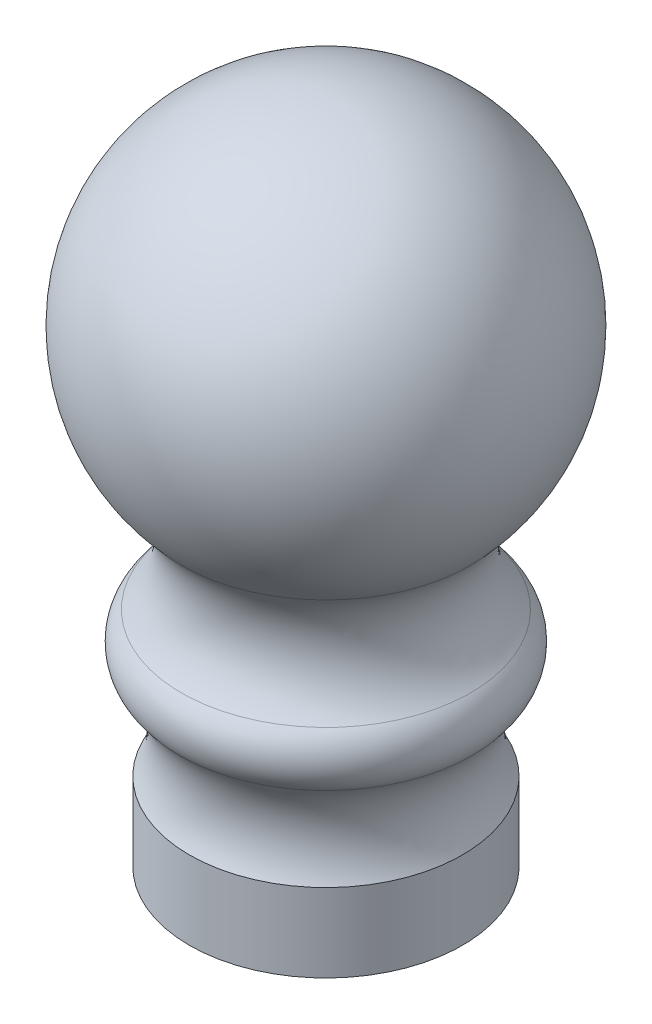
ISO-10303-21;
HEADER;
FILE_DESCRIPTION(('STEP AP214'),'2;1');
FILE_NAME('part.step','',(''),(''),'','','');
FILE_SCHEMA(('AUTOMOTIVE_DESIGN { 1 0 10303 214 1 1 1 1 }'));
ENDSEC;
DATA;
#1=APPLICATION_CONTEXT('core data for automotive mechanical design processes');
#2=APPLICATION_PROTOCOL_DEFINITION('international standard','automotive_design',2000,#1);
#3=PRODUCT_CONTEXT('',#1,'mechanical');
#4=PRODUCT('Part','Part','',(#3));
#5=PRODUCT_RELATED_PRODUCT_CATEGORY('part','',(#4));
#6=PRODUCT_DEFINITION_FORMATION('','',#4);
#7=PRODUCT_DEFINITION_CONTEXT('part definition',#1,'design');
#8=PRODUCT_DEFINITION('design','',#6,#7);
#9=PRODUCT_DEFINITION_SHAPE('','',#8);
#10=(LENGTH_UNIT() NAMED_UNIT(*) SI_UNIT(.MILLI.,.METRE.));
#11=(NAMED_UNIT(*) PLANE_ANGLE_UNIT() SI_UNIT($,.RADIAN.));
#12=(NAMED_UNIT(*) SI_UNIT($,.STERADIAN.) SOLID_ANGLE_UNIT());
#13=UNCERTAINTY_MEASURE_WITH_UNIT(LENGTH_MEASURE(1.E-05),#10,'distance_accuracy_value','');
#14=(GEOMETRIC_REPRESENTATION_CONTEXT(3) GLOBAL_UNCERTAINTY_ASSIGNED_CONTEXT((#13)) GLOBAL_UNIT_ASSIGNED_CONTEXT((#10,
#11,#12)) REPRESENTATION_CONTEXT('',''));
#15=CARTESIAN_POINT('',(0.,0.,0.));
#16=DIRECTION('',(0.,0.,1.));
#17=DIRECTION('',(1.,0.,0.));
#18=AXIS2_PLACEMENT_3D('',#15,#16,#17);
#19=CARTESIAN_POINT('',(0.,24.,0.));
#20=DIRECTION('',(0.,-1.,0.));
#21=DIRECTION('',(1.,0.,0.));
#22=AXIS2_PLACEMENT_3D('',#19,#20,#21);
#23=SPHERICAL_SURFACE('',#22,10.147938904834);
#24=CARTESIAN_POINT('',(0.,24.,-9.32634247796231));
#25=DIRECTION('',(0.,0.,1.));
#26=DIRECTION('',(1.,0.,0.));
#27=AXIS2_PLACEMENT_3D('',#24,#25,#26);
#28=CIRCLE('',#27,4.);
#29=CARTESIAN_POINT('',(4.,24.,-9.32634247796231));
#30=VERTEX_POINT('',#29);
#31=EDGE_CURVE('E44',#30,#30,#28,.T.);
#32=ORIENTED_EDGE('',*,*,#31,.T.);
#33=EDGE_LOOP('',(#32));
#34=FACE_BOUND('',#33,.T.);
#35=CARTESIAN_POINT('',(0.,17.0710678118655,0.));
#36=DIRECTION('',(0.,-1.,0.));
#37=DIRECTION('',(0.,0.,-1.));
#38=AXIS2_PLACEMENT_3D('',#35,#36,#37);
#39=CIRCLE('',#38,7.4142135623731);
#40=CARTESIAN_POINT('',(0.,17.0710678118655,-7.4142135623731));
#41=VERTEX_POINT('',#40);
#42=EDGE_CURVE('E11',#41,#41,#39,.T.);
#43=ORIENTED_EDGE('',*,*,#42,.F.);
#44=EDGE_LOOP('',(#43));
#45=FACE_BOUND('',#44,.T.);
#46=CARTESIAN_POINT('',(-9.32634247796231,24.,0.));
#47=DIRECTION('',(1.,0.,0.));
#48=DIRECTION('',(0.,0.,-1.));
#49=AXIS2_PLACEMENT_3D('',#46,#47,#48);
#50=CIRCLE('',#49,4.);
#51=CARTESIAN_POINT('',(-9.32634247796231,24.,-4.));
#52=VERTEX_POINT('',#51);
#53=EDGE_CURVE('E98',#52,#52,#50,.T.);
#54=ORIENTED_EDGE('',*,*,#53,.T.);
#55=EDGE_LOOP('',(#54));
#56=FACE_BOUND('',#55,.T.);
#57=ADVANCED_FACE('F41',(#34,#45,#56),#23,.T.);
#58=CARTESIAN_POINT('',(0.,24.,4.));
#59=DIRECTION('',(0.,0.,-1.));
#60=DIRECTION('',(-1.,0.,0.));
#61=AXIS2_PLACEMENT_3D('',#58,#59,#60);
#62=CYLINDRICAL_SURFACE('',#61,4.);
#63=ORIENTED_EDGE('',*,*,#31,.F.);
#64=EDGE_LOOP('',(#63));
#65=FACE_BOUND('',#64,.T.);
#66=CARTESIAN_POINT('',(0.,24.,0.));
#67=DIRECTION('',(0.707106781186547,0.,-0.707106781186547));
#68=DIRECTION('',(-0.707106781186547,0.,-0.707106781186547));
#69=AXIS2_PLACEMENT_3D('',#66,#67,#68);
#70=ELLIPSE('',#69,5.65685424949238,4.);
#71=CARTESIAN_POINT('',(0.,28.,0.));
#72=VERTEX_POINT('',#71);
#73=CARTESIAN_POINT('',(0.,20.,0.));
#74=VERTEX_POINT('',#73);
#75=EDGE_CURVE('E60',#72,#74,#70,.F.);
#76=ORIENTED_EDGE('',*,*,#75,.T.);
#77=CARTESIAN_POINT('',(0.,24.,0.));
#78=DIRECTION('',(-0.707106781186547,0.,-0.707106781186547));
#79=DIRECTION('',(0.707106781186547,0.,-0.707106781186547));
#80=AXIS2_PLACEMENT_3D('',#77,#78,#79);
#81=ELLIPSE('',#80,5.65685424949238,4.);
#82=CARTESIAN_POINT('',(4.,24.,-4.));
#83=VERTEX_POINT('',#82);
#84=EDGE_CURVE('E76',#74,#83,#81,.F.);
#85=ORIENTED_EDGE('',*,*,#84,.T.);
#86=EDGE_CURVE('E71',#83,#72,#81,.F.);
#87=ORIENTED_EDGE('',*,*,#86,.T.);
#88=EDGE_LOOP('',(#76,#85,#87));
#89=FACE_BOUND('',#88,.T.);
#90=ADVANCED_FACE('F95',(#65,#89),#62,.F.);
#91=CARTESIAN_POINT('',(0.,14.2426406871193,0.));
#92=DIRECTION('',(0.,-1.,0.));
#93=DIRECTION('',(0.,0.,-1.));
#94=AXIS2_PLACEMENT_3D('',#91,#92,#93);
#95=TOROIDAL_SURFACE('',#94,10.2426406871193,4.);
#96=ORIENTED_EDGE('',*,*,#42,.T.);
#97=EDGE_LOOP('',(#96));
#98=FACE_BOUND('',#97,.T.);
#99=CARTESIAN_POINT('',(0.,11.4142135623731,0.));
#100=DIRECTION('',(0.,-1.,0.));
#101=DIRECTION('',(0.,0.,-1.));
#102=AXIS2_PLACEMENT_3D('',#99,#100,#101);
#103=CIRCLE('',#102,7.4142135623731);
#104=CARTESIAN_POINT('',(0.,11.4142135623731,-7.4142135623731));
#105=VERTEX_POINT('',#104);
#106=EDGE_CURVE('E104',#105,#105,#103,.T.);
#107=ORIENTED_EDGE('',*,*,#106,.F.);
#108=EDGE_LOOP('',(#107));
#109=FACE_BOUND('',#108,.T.);
#110=ADVANCED_FACE('F43',(#98,#109),#95,.F.);
#111=CARTESIAN_POINT('',(0.,0.,0.));
#112=DIRECTION('',(0.,-1.,0.));
#113=DIRECTION('',(0.,0.,-1.));
#114=AXIS2_PLACEMENT_3D('',#111,#112,#113);
#115=PLANE('',#114);
#116=CARTESIAN_POINT('',(0.,0.,0.));
#117=DIRECTION('',(0.,-1.,0.));
#118=DIRECTION('',(0.,0.,-1.));
#119=AXIS2_PLACEMENT_3D('',#116,#117,#118);
#120=CIRCLE('',#119,7.);
#121=CARTESIAN_POINT('',(0.,0.,-7.));
#122=VERTEX_POINT('',#121);
#123=EDGE_CURVE('E49',#122,#122,#120,.T.);
#124=ORIENTED_EDGE('',*,*,#123,.T.);
#125=EDGE_LOOP('',(#124));
#126=FACE_BOUND('',#125,.T.);
#127=ADVANCED_FACE('F119',(#126),#115,.T.);
#128=CARTESIAN_POINT('',(0.,0.,0.));
#129=DIRECTION('',(0.,-1.,0.));
#130=DIRECTION('',(0.,0.,-1.));
#131=AXIS2_PLACEMENT_3D('',#128,#129,#130);
#132=CYLINDRICAL_SURFACE('',#131,7.);
#133=CARTESIAN_POINT('',(0.,4.01398088881321,0.));
#134=DIRECTION('',(0.,-1.,0.));
#135=DIRECTION('',(0.,0.,-1.));
#136=AXIS2_PLACEMENT_3D('',#133,#134,#135);
#137=CIRCLE('',#136,7.);
#138=CARTESIAN_POINT('',(0.,4.01398088881321,-7.));
#139=VERTEX_POINT('',#138);
#140=EDGE_CURVE('E112',#139,#139,#137,.T.);
#141=ORIENTED_EDGE('',*,*,#140,.T.);
#142=EDGE_LOOP('',(#141));
#143=FACE_BOUND('',#142,.T.);
#144=ORIENTED_EDGE('',*,*,#123,.F.);
#145=EDGE_LOOP('',(#144));
#146=FACE_BOUND('',#145,.T.);
#147=ADVANCED_FACE('F116',(#143,#146),#132,.T.);
#148=CARTESIAN_POINT('',(0.,6.,0.));
#149=DIRECTION('',(0.,-1.,0.));
#150=DIRECTION('',(0.,0.,-1.));
#151=AXIS2_PLACEMENT_3D('',#148,#149,#150);
#152=TOROIDAL_SURFACE('',#151,10.4721359549996,4.);
#153=CARTESIAN_POINT('',(0.,8.66666666666667,0.));
#154=DIRECTION('',(0.,-1.,0.));
#155=DIRECTION('',(0.,0.,-1.));
#156=AXIS2_PLACEMENT_3D('',#153,#154,#155);
#157=CIRCLE('',#156,7.49071198499986);
#158=CARTESIAN_POINT('',(0.,8.66666666666667,-7.49071198499986));
#159=VERTEX_POINT('',#158);
#160=EDGE_CURVE('E107',#159,#159,#157,.T.);
#161=ORIENTED_EDGE('',*,*,#160,.T.);
#162=EDGE_LOOP('',(#161));
#163=FACE_BOUND('',#162,.T.);
#164=ORIENTED_EDGE('',*,*,#140,.F.);
#165=EDGE_LOOP('',(#164));
#166=FACE_BOUND('',#165,.T.);
#167=ADVANCED_FACE('F122',(#163,#166),#152,.F.);
#168=CARTESIAN_POINT('',(0.,10.,0.));
#169=DIRECTION('',(0.,-1.,0.));
#170=DIRECTION('',(0.,0.,-1.));
#171=AXIS2_PLACEMENT_3D('',#168,#169,#170);
#172=TOROIDAL_SURFACE('',#171,6.,2.);
#173=ORIENTED_EDGE('',*,*,#106,.T.);
#174=EDGE_LOOP('',(#173));
#175=FACE_BOUND('',#174,.T.);
#176=ORIENTED_EDGE('',*,*,#160,.F.);
#177=EDGE_LOOP('',(#176));
#178=FACE_BOUND('',#177,.T.);
#179=ADVANCED_FACE('F126',(#175,#178),#172,.T.);
#180=CARTESIAN_POINT('',(4.,24.,0.));
#181=DIRECTION('',(-1.,0.,0.));
#182=DIRECTION('',(0.,0.,1.));
#183=AXIS2_PLACEMENT_3D('',#180,#181,#182);
#184=CYLINDRICAL_SURFACE('',#183,4.);
#185=ORIENTED_EDGE('',*,*,#53,.F.);
#186=EDGE_LOOP('',(#185));
#187=FACE_BOUND('',#186,.T.);
#188=CARTESIAN_POINT('',(0.,24.,0.));
#189=DIRECTION('',(-0.707106781186547,0.,-0.707106781186547));
#190=DIRECTION('',(0.707106781186547,0.,-0.707106781186547));
#191=AXIS2_PLACEMENT_3D('',#188,#189,#190);
#192=ELLIPSE('',#191,5.65685424949238,4.);
#193=CARTESIAN_POINT('',(-4.,24.,4.));
#194=VERTEX_POINT('',#193);
#195=EDGE_CURVE('E92',#194,#72,#192,.T.);
#196=ORIENTED_EDGE('',*,*,#195,.F.);
#197=EDGE_CURVE('E78',#74,#194,#192,.T.);
#198=ORIENTED_EDGE('',*,*,#197,.F.);
#199=ORIENTED_EDGE('',*,*,#75,.F.);
#200=EDGE_LOOP('',(#196,#198,#199));
#201=FACE_BOUND('',#200,.T.);
#202=ADVANCED_FACE('F149',(#187,#201),#184,.F.);
#203=CARTESIAN_POINT('',(0.,24.,4.));
#204=DIRECTION('',(0.,0.,1.));
#205=DIRECTION('',(1.,0.,0.));
#206=AXIS2_PLACEMENT_3D('',#203,#204,#205);
#207=PLANE('',#206);
#208=CARTESIAN_POINT('',(0.,24.,4.));
#209=DIRECTION('',(0.,0.,1.));
#210=DIRECTION('',(1.,0.,0.));
#211=AXIS2_PLACEMENT_3D('',#208,#209,#210);
#212=CIRCLE('',#211,4.);
#213=CARTESIAN_POINT('',(4.,24.,4.));
#214=VERTEX_POINT('',#213);
#215=EDGE_CURVE('E101',#194,#214,#212,.T.);
#216=ORIENTED_EDGE('',*,*,#215,.F.);
#217=EDGE_CURVE('E105',#214,#194,#212,.T.);
#218=ORIENTED_EDGE('',*,*,#217,.F.);
#219=EDGE_LOOP('',(#216,#218));
#220=FACE_BOUND('',#219,.T.);
#221=ADVANCED_FACE('F155',(#220),#207,.F.);
#222=CARTESIAN_POINT('',(0.,24.,0.));
#223=DIRECTION('',(0.707106781186547,0.,-0.707106781186547));
#224=DIRECTION('',(-0.707106781186547,0.,-0.707106781186547));
#225=AXIS2_PLACEMENT_3D('',#222,#223,#224);
#226=ELLIPSE('',#225,5.65685424949238,4.);
#227=EDGE_CURVE('E86',#214,#74,#226,.T.);
#228=ORIENTED_EDGE('',*,*,#227,.T.);
#229=ORIENTED_EDGE('',*,*,#197,.T.);
#230=ORIENTED_EDGE('',*,*,#215,.T.);
#231=EDGE_LOOP('',(#228,#229,#230));
#232=FACE_BOUND('',#231,.T.);
#233=ADVANCED_FACE('F136',(#232),#62,.F.);
#234=ORIENTED_EDGE('',*,*,#195,.T.);
#235=EDGE_CURVE('E63',#72,#214,#226,.T.);
#236=ORIENTED_EDGE('',*,*,#235,.T.);
#237=ORIENTED_EDGE('',*,*,#217,.T.);
#238=EDGE_LOOP('',(#234,#236,#237));
#239=FACE_BOUND('',#238,.T.);
#240=ADVANCED_FACE('F143',(#239),#62,.F.);
#241=ORIENTED_EDGE('',*,*,#227,.F.);
#242=CARTESIAN_POINT('',(4.,24.,0.));
#243=DIRECTION('',(1.,0.,0.));
#244=DIRECTION('',(0.,0.,-1.));
#245=AXIS2_PLACEMENT_3D('',#242,#243,#244);
#246=CIRCLE('',#245,4.);
#247=EDGE_CURVE('E81',#214,#83,#246,.T.);
#248=ORIENTED_EDGE('',*,*,#247,.T.);
#249=ORIENTED_EDGE('',*,*,#84,.F.);
#250=EDGE_LOOP('',(#241,#248,#249));
#251=FACE_BOUND('',#250,.T.);
#252=ADVANCED_FACE('F88',(#251),#184,.F.);
#253=CARTESIAN_POINT('',(4.,24.,0.));
#254=DIRECTION('',(1.,0.,0.));
#255=DIRECTION('',(0.,0.,-1.));
#256=AXIS2_PLACEMENT_3D('',#253,#254,#255);
#257=PLANE('',#256);
#258=EDGE_CURVE('E79',#83,#214,#246,.T.);
#259=ORIENTED_EDGE('',*,*,#258,.F.);
#260=ORIENTED_EDGE('',*,*,#247,.F.);
#261=EDGE_LOOP('',(#259,#260));
#262=FACE_BOUND('',#261,.T.);
#263=ADVANCED_FACE('F93',(#262),#257,.F.);
#264=ORIENTED_EDGE('',*,*,#86,.F.);
#265=ORIENTED_EDGE('',*,*,#258,.T.);
#266=ORIENTED_EDGE('',*,*,#235,.F.);
#267=EDGE_LOOP('',(#264,#265,#266));
#268=FACE_BOUND('',#267,.T.);
#269=ADVANCED_FACE('F73',(#268),#184,.F.);
#270=CLOSED_SHELL('',(#57,#90,#110,#127,#147,#167,#179,#202,#221,#233,#240,#252,#263,#269));
#271=MANIFOLD_SOLID_BREP('B2',#270);
#272=ADVANCED_BREP_SHAPE_REPRESENTATION('',(#18,#271),#14);
#273=SHAPE_DEFINITION_REPRESENTATION(#9,#272);
ENDSEC;
END-ISO-10303-21;
